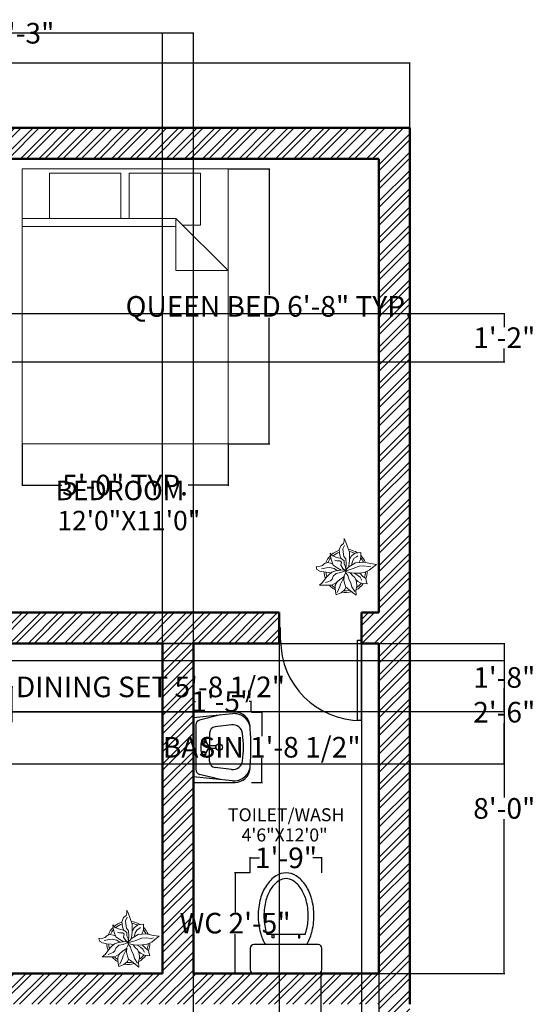
# Model space of a CAD drawing. Units: inches. Extents: x -71 to 434, y -519 to 67.
# Tile 7 of 7: x 270 to 420, y -224 to 62. Entities that reach past the tile are written whole.
import ezdxf

# ---------------------------------------------------------------- set-up
doc = ezdxf.new("R2010")
doc.units = ezdxf.units.IN
doc.header["$MEASUREMENT"] = 0
for name, color, linetype, lineweight in [('A-ANNO-DIMS', 7, 'Continuous', 18), ('A-AREA-IDEN', 7, 'Continuous', 25), ('A-FLOR-FIXT', 9, 'Continuous', 18), ('A-WALL-PATT', 8, 'Continuous', 13), ('CAY', 94, 'Continuous', 13), ('DOOR', 3, 'Continuous', 25), ('FURNITURE', 5, 'Continuous', 18), ('WALL', 50, 'Continuous', 50)]:
    doc.layers.add(name, color=color, linetype=linetype, lineweight=lineweight)
doc.layers.add('THIET-BI', color=21, linetype='Continuous')
doc.styles.add('ATT', font='romans.shx')
doc.styles.get("Standard").update_dxf_attribs({"font": 'arial.ttf'})
doc.dimstyles.get("Standard").update_dxf_attribs({"dimtxt": 6, "dimasz": 0.18, "dimexe": 0.18, "dimexo": 0.0625, "dimgap": 0.09, "dimtad": 0, "dimtih": 1, "dimtoh": 1, "dimdec": 0, "dimzin": 0, "dimdsep": 46, "dimlunit": 3, "dimtxsty": 'Standard', "dimcen": 0.09, "dimadec": 0, "dimazin": 0, "dimtfac": 1, "dimtdec": 0, "dimtofl": 0, "dimtmove": 0, "dimatfit": 3, "dimfxl": 1, "dimtolj": 1, "dimtzin": 0, "dimarcsym": 0})

# ---------------------------------------------------------------- blocks, each defined once
blk = doc.blocks.new('Bed - Queen')
for p, q in [((0, -80.00003), (0, 0)), ((0, 0), (59.99999, 0)), ((59.99999, 0), (59.99999, -80.00003)), ((7.99999, -1.2), (28.79998, -1.2)), ((7.99999, -14.4), (7.99999, -1.2)), ((28.79998, -1.2), (28.79998, -14.4)), ((31.19999, -1.2), (51.99999, -1.2)), ((31.19999, -14.4), (31.19999, -1.2)), ((51.99999, -1.2), (51.99999, -16.4)), ((0, -14.4), (44.8, -14.4)), ((44.8, -16.8), (0, -16.8)), ((59.99999, -29.6), (44.8, -14.4)), ((44.8, -14.4), (44.8, -29.6)), ((51.99999, -16.4), (46.79936, -16.4)), ((44.8, -29.6), (59.99999, -29.6)), ((59.99999, -80.00003), (0, -80.00003))]:
    blk.add_line(p, q)
blk = doc.blocks.new('A$C793314D9')
at = {"layer": 'THIET-BI'}
for p, q in [((475, 700), (25, 700)), ((0, 675), (0, 525)), ((500, 525), (500, 675)), ((25, 500), (475, 500)), ((117.1, 430), (382.9, 430)), ((163.6, 452.4), (153.8, 452.4)), ((153.8, 452.4), (153.8, 429.9)), ((153.8, 429.9), (163.6, 429.9)), ((163.6, 429.9), (163.6, 452.4)), ((336.2, 452.4), (345.9, 452.4)), ((336.2, 429.9), (336.2, 452.4)), ((345.9, 429.9), (336.2, 429.9)), ((345.9, 452.4), (345.9, 429.9))]:
    blk.add_line(p, q, dxfattribs=at)
for centre, radius, start, end in [((25, 675), 25, 90, 180), ((475, 675), 25, 0, 90), ((25, 525), 25, 180, 270), ((383.8, 333.9), 323.5, 149.09657, 164.92686), ((116.2, 333.9), 323.5, 15.07314, 30.90343), ((475, 525), 25, 270, 0), ((513.7, 298.9), 458.1, 164.92686, 180), ((383.8, 333.9), 283.5, 160.17598, 164.92686), ((116.2, 333.9), 283.5, 15.07314, 19.82402), ((-13.7, 298.9), 458.1, 0, 15.07314), ((513.7, 298.9), 418.1, 164.92686, 180), ((-13.7, 298.9), 418.1, 0, 15.07314), ((513.7, 298.9), 458.1, 180, 195.07314), ((513.7, 298.9), 418.1, 180, 195.07314), ((-13.7, 298.9), 418.1, 344.92686, 360), ((-13.7, 298.9), 458.1, 344.92686, 0), ((383.8, 263.9), 323.5, 195.07314, 213.03155), ((383.8, 263.9), 283.5, 195.07314, 213.03155), ((116.2, 263.9), 283.5, 326.96845, 344.92686), ((116.2, 263.9), 323.5, 326.96845, 344.92686), ((301.7, 210.5), 225.5, 213.03155, 237.50023), ((301.7, 210.5), 185.5, 213.03155, 237.50023), ((198.3, 210.5), 185.5, 302.49977, 326.96845), ((198.3, 210.5), 225.5, 302.49977, 326.96845), ((250, 129.3), 129.3, 237.50023, 270), ((250, 129.3), 89.3, 237.50023, 270), ((250, 129.3), 89.3, 270, 302.49977), ((250, 129.3), 129.3, 270, 302.49977)]:
    blk.add_arc(centre, radius, start, end, dxfattribs=at)
blk = doc.blocks.new('TAM')
for p, q in [((-68.4, 12), (-49.4, 25.8)), ((-61.2, -10.4), (-68.4, 12)), ((-59.4, 6.8), (-61.2, 6.8)), ((-49.4, 25.8), (-30.4, 12)), ((-30.4, 12), (-37.6, -10.4)), ((50.6, 25.8), (31.6, 12)), ((31.6, 12), (38.8, -10.4)), ((69.6, 12), (50.6, 25.8)), ((60.6, 6.8), (62.4, 6.8)), ((62.4, -10.4), (69.6, 12)), ((-59.4, -10.4), (-49.4, -10.4)), ((-9.4, -60.4), (-9.4, -50.4)), ((-9.4, -90.4), (-9.4, -60.4)), ((10.6, -60.4), (10.6, -50.4)), ((10.6, -90.4), (10.6, -60.4)), ((62.4, -10.4), (50.6, -10.4)), ((-9.4, -90.4), (10.6, -90.4))]:
    blk.add_line(p, q)
for centre in [(-49.8, 6.8), (51, 6.8)]:
    blk.add_circle(centre, 10.4)
for centre, radius, start, end in [((0.6, -221.7), 252.5, 78.57881, 101.42119), ((-49.4, -50.4), 40, 0, 90), ((50.6, -50.4), 40, 90, 180)]:
    blk.add_arc(centre, radius, start, end)
blk = doc.blocks.new('A$C0E2F1A29')
at = {"layer": 'THIET-BI'}
for p, q in [((0, 460), (0, 126.9)), ((560, 460), (0, 460)), ((13, 148.3), (44.6, 460)), ((22.6, 242.8), (63.6, 409.5)), ((457.6, 440), (102.4, 440)), ((537.4, 242.8), (496.4, 409.5)), ((547, 148.3), (515.4, 460)), ((560, 126.9), (560, 460)), ((167.1, 330), (280, 330)), ((392.9, 330), (280, 330)), ((101.6, 155.5), (117.4, 286)), ((458.4, 155.5), (442.6, 286))]:
    blk.add_line(p, q, dxfattribs=at)
blk.add_circle((280, 253.2), 25.4, dxfattribs=at)
for centre, radius, start, end in [((102.4, 400), 40, 90, 166.19533), ((457.6, 400), 40, 13.80467, 90), ((167.1, 280), 50, 90, 173.07801), ((392.9, 280), 50, 6.92199, 90), ((120, 126.9), 120, 180, 265.03849), ((142.3, 135.2), 130, 174.2113, 265.70941), ((181, 145.9), 80, 173.07801, 263.17143), ((379, 145.9), 80, 276.82857, 6.92199), ((417.7, 135.2), 130, 274.29059, 5.7887), ((440, 126.9), 120, 274.96151, 0), ((280, 1970), 1970, 265.70941, 274.29059), ((280, 972.5), 912.5, 263.17143, 276.82857)]:
    blk.add_arc(centre, radius, start, end, dxfattribs=at)
blk.add_blockref('TAM', (279.2, 369.4), dxfattribs=at)
blk = doc.blocks.new('*U13')
for p, q in [((0, 0), (0, -6)), ((40, 0), (40, -6))]:
    blk.add_line(p, q)
blk.add_lwpolyline([(0, 0), (0, 40), (1.75, 40), (1.75, 0)], close=True)
blk.add_arc((0, 0), 40, 0, 90)
blk = doc.blocks.new('*D17')
at = {"layer": 'A-ANNO-DIMS', "color": 0, "lineweight": -2, "transparency": 16777216}
for p, q in [((-12.59, 30.9), (-12.59, 49.86)), ((-12.41, 49.68), (180.23, 49.68)), ((383.23, 49.68), (190.59, 49.68)), ((383.41, 30.9), (383.41, 49.86))]:
    blk.add_line(p, q, dxfattribs=at)
at = {"layer": 'A-ANNO-DIMS', "color": 0, "transparency": 16777216}
for points in [[(-12.41, 49.71), (-12.41, 49.65), (-12.59, 49.68)], [(383.23, 49.71), (383.23, 49.65), (383.41, 49.68)]]:
    blk.add_solid(points, dxfattribs=at)
at = {"layer": 'Defpoints', "color": 0, "transparency": 16777216}
for p in [(383.41, 49.68), (-12.59, 30.83), (383.41, 30.83)]:
    blk.add_point(p, dxfattribs=at)
at = {"layer": 'A-ANNO-DIMS', "color": 0, "transparency": 16777216, "insert": (185.41, 49.68), "char_height": 6, "attachment_point": 5}
blk.add_mtext("\\A1;33'", dxfattribs=at)
blk = doc.blocks.new('12PPLT12')
at = {"color": 0, "linetype": 'ByBlock'}
for p, q in [((-0.05, 0.632), (-0.034, 0.694)), ((-0.034, 0.694), (-0.032, 0.751)), ((-0.032, 0.751), (-0.002, 0.689)), ((-0.002, 0.689), (0.044, 0.559)), ((-0.148, 0.486), (-0.116, 0.583)), ((-0.132, 0.367), (-0.148, 0.486)), ((-0.116, 0.583), (-0.05, 0.632)), ((-0.064, 0.51), (-0.026, 0.591)), ((-0.05, 0.38), (-0.064, 0.51)), ((0.044, 0.559), (0.09, 0.432)), ((-0.349, 0.334), (-0.362, 0.415)), ((-0.362, 0.415), (-0.303, 0.35)), ((-0.332, 0.247), (-0.349, 0.334)), ((-0.289, 0.136), (-0.332, 0.247)), ((-0.303, 0.35), (-0.208, 0.312)), ((-0.205, 0.231), (-0.251, 0.247)), ((-0.208, 0.312), (-0.105, 0.29)), ((-0.137, 0.231), (-0.205, 0.231)), ((-0.097, 0.204), (-0.137, 0.231)), ((-0.108, 0.279), (-0.132, 0.367)), ((-0.105, 0.29), (-0.037, 0.236)), ((-0.043, 0.334), (-0.05, 0.38)), ((0.003, 0.279), (-0.043, 0.334)), ((-0.037, 0.236), (-0.034, 0.158)), ((0.009, 0.169), (0.003, 0.279)), ((0.09, 0.253), (0.082, 0.174)), ((0.09, 0.432), (0.09, 0.339)), ((0.09, 0.339), (0.09, 0.253)), ((0.093, 0.282), (0.134, 0.347)), ((0.155, 0.228), (0.131, 0.13)), ((0.134, 0.347), (0.22, 0.415)), ((0.193, 0.293), (0.155, 0.228)), ((0.25, 0.328), (0.193, 0.293)), ((0.22, 0.415), (0.291, 0.421)), ((0.28, 0.353), (0.25, 0.328)), ((0.291, 0.421), (0.35, 0.429)), ((0.342, 0.266), (0.304, 0.19)), ((0.348, 0.331), (0.342, 0.266)), ((0.35, 0.429), (0.348, 0.331)), ((-0.671, 0.098), (-0.687, 0.095)), ((-0.687, 0.095), (-0.666, 0.036)), ((-0.59, 0.109), (-0.671, 0.098)), ((-0.666, 0.036), (-0.601, -0.005)), ((-0.536, 0.125), (-0.59, 0.109)), ((-0.563, 0.052), (-0.441, 0.074)), ((-0.487, 0.171), (-0.536, 0.125)), ((-0.425, 0.193), (-0.487, 0.171)), ((-0.441, 0.074), (-0.373, 0.084)), ((-0.346, 0.179), (-0.425, 0.193)), ((-0.373, 0.084), (-0.27, 0.057)), ((-0.292, 0.149), (-0.346, 0.179)), ((-0.229, 0.003), (-0.324, -0.027)), ((-0.194, 0.074), (-0.289, 0.136)), ((-0.27, 0.057), (-0.186, 0.006)), ((-0.069, 0.027), (-0.229, 0.003)), ((-0.108, 0.019), (-0.194, 0.074)), ((-0.01, 0.003), (-0.121, -0.038)), ((-0.11, 0.133), (-0.097, 0.204)), ((-0.069, 0.06), (-0.11, 0.133)), ((-0.01, 0.014), (-0.069, 0.06)), ((-0.002, 0.006), (-0.069, 0.027)), ((-0.034, 0.158), (-0.007, 0.101)), ((-0.018, -0.008), (0.074, 0.098)), ((-0.01, -0.005), (0.169, 0.055)), ((0.003, 0.017), (-0.01, 0.014)), ((0.003, -0.029), (-0.01, 0.003)), ((-0.007, 0.101), (0.003, 0.017)), ((0.006, 0.027), (0.009, 0.169)), ((0.082, 0.174), (0.061, 0.082)), ((0.074, 0.098), (0.223, 0.188)), ((0.169, 0.055), (0.315, 0.109)), ((0.223, 0.188), (0.421, 0.204)), ((0.315, 0.109), (0.413, 0.117)), ((0.413, 0.117), (0.524, 0.101)), ((0.421, 0.204), (0.573, 0.171)), ((0.545, 0.017), (0.429, -0.032)), ((0.524, 0.101), (0.578, 0.114)), ((0.613, 0.074), (0.545, 0.017)), ((0.573, 0.171), (0.716, 0.152)), ((0.716, 0.152), (0.613, 0.074)), ((-0.601, -0.005), (-0.503, -0.021)), ((-0.452, -0.152), (-0.536, -0.268)), ((-0.503, -0.021), (-0.4, -0.032)), ((-0.395, -0.094), (-0.452, -0.152)), ((-0.4, -0.032), (-0.357, -0.04)), ((-0.324, -0.027), (-0.395, -0.094)), ((-0.352, -0.227), (-0.387, -0.241)), ((-0.316, -0.187), (-0.352, -0.227)), ((-0.292, -0.122), (-0.316, -0.187)), ((-0.224, -0.059), (-0.292, -0.122)), ((-0.121, -0.038), (-0.224, -0.059)), ((-0.213, -0.263), (-0.135, -0.195)), ((-0.135, -0.195), (-0.053, -0.14)), ((-0.119, -0.304), (-0.04, -0.148)), ((-0.053, -0.14), (0.003, -0.029)), ((-0.037, -0.122), (-0.04, -0.219)), ((-0.04, -0.219), (-0.021, -0.308)), ((0.082, -0.038), (-0.018, -0.008)), ((-0.007, -0.024), (0.05, -0.105)), ((0.05, -0.105), (0.071, -0.181)), ((0.071, -0.181), (0.12, -0.282)), ((0.188, -0.054), (0.082, -0.038)), ((0.112, -0.051), (0.09, -0.043)), ((0.155, -0.108), (0.112, -0.051)), ((0.212, -0.152), (0.155, -0.108)), ((0.323, -0.051), (0.188, -0.054)), ((0.247, -0.246), (0.212, -0.152)), ((0.215, -0.062), (0.282, -0.103)), ((0.234, -0.2), (0.277, -0.241)), ((0.282, -0.103), (0.334, -0.146)), ((0.429, -0.032), (0.323, -0.051)), ((0.396, -0.124), (0.326, -0.054)), ((0.334, -0.146), (0.372, -0.217)), ((0.464, -0.176), (0.396, -0.124)), ((0.48, -0.257), (0.464, -0.176)), ((-0.536, -0.268), (-0.606, -0.328)), ((-0.606, -0.328), (-0.522, -0.328)), ((-0.522, -0.328), (-0.324, -0.325)), ((-0.387, -0.241), (-0.465, -0.268)), ((-0.324, -0.325), (-0.213, -0.263)), ((-0.244, -0.33), (-0.247, -0.406)), ((-0.247, -0.406), (-0.233, -0.471)), ((-0.193, -0.236), (-0.244, -0.33)), ((-0.199, -0.494), (-0.139, -0.358)), ((-0.139, -0.358), (-0.119, -0.304)), ((-0.102, -0.503), (-0.017, -0.432)), ((-0.021, -0.308), (0.006, -0.376)), ((-0.017, -0.432), (0.003, -0.378)), ((0.006, -0.376), (0.074, -0.428)), ((0.074, -0.428), (0.158, -0.496)), ((0.12, -0.282), (0.139, -0.363)), ((0.139, -0.363), (0.212, -0.474)), ((0.236, -0.444), (0.261, -0.349)), ((0.242, -0.561), (0.236, -0.444)), ((0.261, -0.349), (0.247, -0.246)), ((0.277, -0.241), (0.372, -0.287)), ((0.372, -0.287), (0.494, -0.301)), ((0.494, -0.301), (0.48, -0.257)), ((-0.233, -0.471), (-0.222, -0.551)), ((-0.222, -0.551), (-0.148, -0.522)), ((-0.148, -0.522), (-0.102, -0.503)), ((0.158, -0.496), (0.242, -0.561))]:
    blk.add_line(p, q, dxfattribs=at)
for radius, start, end in [(0.5, 107.123, 130.9816), (0.5, 56.9563, 82.295), (0.5, 134.8021, 159.1804), (0.458, 138.4756, 155.3347), (0.458, 107.9864, 130.5771), (0.458, 62.6899, 79.5345), (0.458, 26.2761, 41.1349), (0.5, 22.9768, 45.8473), (0.5, 182.503, 200.4563), (0.458, 183.2699, 197.4002), (0.458, 340.6559, 357.5057), (0.5, 338.5862, 359.7442), (0.5, 220.6606, 241.3393), (0.458, 225.0835, 237.5023), (0.458, 264.1886, 282.4028), (0.5, 298.3455, 324.4541), (0.458, 303.3868, 322.0756), (0.5, 259.7038, 286.1281)]:
    blk.add_arc((0, 0), radius, start, end, dxfattribs=at)
at = {"color": 0, "linetype": 'ByBlock', "style": 'ATT'}
for tag, p, flags in [('ITEM', (-1, -3.25), 3), ('ROOM_NUMBER', (-1, -4.583), 1)]:
    blk.add_attdef(tag, p, '', height=1, dxfattribs=dict(at, flags=flags))
blk = doc.blocks.new('*D24')
at = {"layer": 'A-ANNO-DIMS', "color": 0, "lineweight": -2, "transparency": 16777216}
for p, q in [((330.58, 18.91), (342.7, 18.91)), ((342.52, 18.73), (342.52, -17.71)), ((342.52, -60.91), (342.52, -24.46)), ((330.58, -61.09), (342.7, -61.09))]:
    blk.add_line(p, q, dxfattribs=at)
at = {"layer": 'A-ANNO-DIMS', "color": 0, "transparency": 16777216}
for points in [[(342.49, 18.73), (342.55, 18.73), (342.52, 18.91)], [(342.49, -60.91), (342.55, -60.91), (342.52, -61.09)]]:
    blk.add_solid(points, dxfattribs=at)
at = {"layer": 'Defpoints', "color": 0, "transparency": 16777216}
for p in [(330.52, 18.91), (342.52, 18.91), (330.52, -61.09)]:
    blk.add_point(p, dxfattribs=at)
at = {"layer": 'A-ANNO-DIMS', "color": 0, "transparency": 16777216, "insert": (342.52, -21.09), "char_height": 6, "attachment_point": 5}
blk.add_mtext('\\A1;QUEEN BED 6\'-8" TYP.', dxfattribs=at)
blk = doc.blocks.new('*D25')
at = {"layer": 'A-ANNO-DIMS', "color": 0, "lineweight": -2, "transparency": 16777216}
for p, q in [((270.52, -61.15), (270.52, -73.27)), ((330.52, -61.15), (330.52, -73.27)), ((270.7, -73.09), (282.14, -73.09)), ((330.34, -73.09), (318.9, -73.09))]:
    blk.add_line(p, q, dxfattribs=at)
at = {"layer": 'A-ANNO-DIMS', "color": 0, "transparency": 16777216}
for points in [[(270.7, -73.06), (270.7, -73.12), (270.52, -73.09)], [(330.34, -73.06), (330.34, -73.12), (330.52, -73.09)]]:
    blk.add_solid(points, dxfattribs=at)
at = {"layer": 'Defpoints', "color": 0, "transparency": 16777216}
for p in [(270.52, -61.09), (330.52, -61.09), (330.52, -73.09)]:
    blk.add_point(p, dxfattribs=at)
at = {"layer": 'A-ANNO-DIMS', "color": 0, "transparency": 16777216, "insert": (300.52, -73.09), "char_height": 6, "attachment_point": 5}
blk.add_mtext('\\A1;5\'-0" TYP.', dxfattribs=at)
blk = doc.blocks.new('*D28')
at = {"layer": 'A-ANNO-DIMS', "color": 0, "lineweight": -2, "transparency": 16777216}
for p, q in [((336.91, -185.93), (332.4, -185.93)), ((332.58, -186.11), (332.58, -197.36)), ((332.58, -214.99), (332.58, -203.74)), ((336.91, -215.17), (332.4, -215.17))]:
    blk.add_line(p, q, dxfattribs=at)
at = {"layer": 'A-ANNO-DIMS', "color": 0, "transparency": 16777216}
for points in [[(332.55, -186.11), (332.61, -186.11), (332.58, -185.93)], [(332.55, -214.99), (332.61, -214.99), (332.58, -215.17)]]:
    blk.add_solid(points, dxfattribs=at)
at = {"layer": 'Defpoints', "color": 0, "transparency": 16777216}
for p in [(336.97, -185.93), (332.58, -215.17), (336.97, -215.17)]:
    blk.add_point(p, dxfattribs=at)
at = {"layer": 'A-ANNO-DIMS', "color": 0, "transparency": 16777216, "insert": (332.58, -200.55), "char_height": 6, "attachment_point": 5}
blk.add_mtext('\\A1;WC 2\'-5"', dxfattribs=at)
blk = doc.blocks.new('*D29')
at = {"layer": 'A-ANNO-DIMS', "color": 0, "lineweight": -2, "transparency": 16777216}
for p, q in [((336.97, -185.87), (336.97, -181.37)), ((337.15, -181.55), (339.63, -181.55)), ((357.67, -181.55), (355.19, -181.55)), ((357.85, -185.87), (357.85, -181.37))]:
    blk.add_line(p, q, dxfattribs=at)
at = {"layer": 'A-ANNO-DIMS', "color": 0, "transparency": 16777216}
for points in [[(337.15, -181.52), (337.15, -181.58), (336.97, -181.55)], [(357.67, -181.52), (357.67, -181.58), (357.85, -181.55)]]:
    blk.add_solid(points, dxfattribs=at)
at = {"layer": 'Defpoints', "color": 0, "transparency": 16777216}
for p in [(336.97, -181.55), (336.97, -185.93), (357.85, -185.93)]:
    blk.add_point(p, dxfattribs=at)
at = {"layer": 'A-ANNO-DIMS', "color": 0, "transparency": 16777216, "insert": (347.41, -181.55), "char_height": 6, "attachment_point": 5}
blk.add_mtext('\\A1;1\'-9"', dxfattribs=at)
blk = doc.blocks.new('*D34')
at = {"layer": 'A-ANNO-DIMS', "color": 0, "lineweight": -2, "transparency": 16777216}
for p, q in [((337.32, -139.15), (340.51, -139.15)), ((340.33, -139.33), (340.33, -146.17)), ((340.33, -159.4), (340.33, -152.56)), ((337.32, -159.58), (340.51, -159.58))]:
    blk.add_line(p, q, dxfattribs=at)
at = {"layer": 'A-ANNO-DIMS', "color": 0, "transparency": 16777216}
for points in [[(340.3, -139.33), (340.36, -139.33), (340.33, -139.15)], [(340.3, -159.4), (340.36, -159.4), (340.33, -159.58)]]:
    blk.add_solid(points, dxfattribs=at)
at = {"layer": 'Defpoints', "color": 0, "transparency": 16777216}
for p in [(337.26, -139.15), (340.33, -139.15), (337.26, -159.58)]:
    blk.add_point(p, dxfattribs=at)
at = {"layer": 'A-ANNO-DIMS', "color": 0, "transparency": 16777216, "insert": (340.33, -149.37), "char_height": 6, "attachment_point": 5}
blk.add_mtext('\\A1;BASIN 1\'-8 1/2"', dxfattribs=at)
blk = doc.blocks.new('*D35')
at = {"layer": 'A-ANNO-DIMS', "color": 0, "lineweight": -2, "transparency": 16777216}
for p, q in [((320.41, -139.09), (320.41, -135.9)), ((320.59, -136.08), (321.05, -136.08)), ((337.08, -136.08), (336.62, -136.08)), ((337.26, -139.09), (337.26, -135.9))]:
    blk.add_line(p, q, dxfattribs=at)
at = {"layer": 'A-ANNO-DIMS', "color": 0, "transparency": 16777216}
for points in [[(320.59, -136.05), (320.59, -136.11), (320.41, -136.08)], [(337.08, -136.05), (337.08, -136.11), (337.26, -136.08)]]:
    blk.add_solid(points, dxfattribs=at)
at = {"layer": 'Defpoints', "color": 0, "transparency": 16777216}
for p in [(320.41, -136.08), (320.41, -139.15), (337.26, -139.15)]:
    blk.add_point(p, dxfattribs=at)
at = {"layer": 'A-ANNO-DIMS', "color": 0, "transparency": 16777216, "insert": (328.83, -136.08), "char_height": 6, "attachment_point": 5}
blk.add_mtext('\\A1;1\'-5"', dxfattribs=at)
blk = doc.blocks.new('*D42')
at = {"layer": 'A-ANNO-DIMS', "color": 0, "lineweight": -2, "transparency": 16777216}
for p, q in [((199.01, -142.05), (199.01, -131.63)), ((267.7, -142.05), (267.7, -131.63)), ((199.19, -131.81), (267.52, -131.81)), ((267.7, -131.81), (267.88, -131.81))]:
    blk.add_line(p, q, dxfattribs=at)
at = {"layer": 'A-ANNO-DIMS', "color": 0, "transparency": 16777216}
for points in [[(199.19, -131.78), (199.19, -131.84), (199.01, -131.81)], [(267.52, -131.78), (267.52, -131.84), (267.7, -131.81)]]:
    blk.add_solid(points, dxfattribs=at)
at = {"layer": 'Defpoints', "color": 0, "transparency": 16777216}
for p in [(267.7, -131.81), (199.01, -142.12), (267.7, -142.12)]:
    blk.add_point(p, dxfattribs=at)
at = {"layer": 'A-ANNO-DIMS', "color": 0, "transparency": 16777216, "insert": (307.94, -131.81), "char_height": 6, "attachment_point": 5}
blk.add_mtext('\\A1;DINING SET 5\'-8 1/2"', dxfattribs=at)
blk = doc.blocks.new('*D49')
at = {"layer": 'A-ANNO-DIMS', "color": 0, "lineweight": -2, "transparency": 16777216}
for p, q in [((221.41, -473.1), (221.41, 58.56)), ((221.59, 58.38), (262.84, 58.38)), ((320.23, 58.38), (278.98, 58.38)), ((320.41, -473.1), (320.41, 58.56))]:
    blk.add_line(p, q, dxfattribs=at)
at = {"layer": 'A-ANNO-DIMS', "color": 0, "transparency": 16777216}
for points in [[(221.59, 58.41), (221.59, 58.35), (221.41, 58.38)], [(320.23, 58.41), (320.23, 58.35), (320.41, 58.38)]]:
    blk.add_solid(points, dxfattribs=at)
at = {"layer": 'Defpoints', "color": 0, "transparency": 16777216}
for p in [(320.41, 58.38), (221.41, -473.17), (320.41, -473.17)]:
    blk.add_point(p, dxfattribs=at)
at = {"layer": 'A-ANNO-DIMS', "color": 0, "transparency": 16777216, "insert": (270.91, 58.38), "char_height": 6, "attachment_point": 5}
blk.add_mtext('\\A1;8\'-3"', dxfattribs=at)
blk = doc.blocks.new('*D53')
at = {"layer": 'A-ANNO-DIMS', "color": 0, "lineweight": -2, "transparency": 16777216}
for p, q in [((374.47, -119.17), (411.14, -119.17)), ((410.96, -119.35), (410.96, -164.01)), ((410.96, -214.99), (410.96, -170.32)), ((374.47, -215.17), (411.14, -215.17))]:
    blk.add_line(p, q, dxfattribs=at)
at = {"layer": 'A-ANNO-DIMS', "color": 0, "transparency": 16777216}
for points in [[(410.93, -119.35), (410.99, -119.35), (410.96, -119.17)], [(410.93, -214.99), (410.99, -214.99), (410.96, -215.17)]]:
    blk.add_solid(points, dxfattribs=at)
at = {"layer": 'Defpoints', "color": 0, "transparency": 16777216}
for p in [(374.41, -119.17), (374.41, -215.17), (410.96, -215.17)]:
    blk.add_point(p, dxfattribs=at)
at = {"layer": 'A-ANNO-DIMS', "color": 0, "transparency": 16777216, "insert": (410.96, -167.17), "char_height": 6, "attachment_point": 5}
blk.add_mtext('\\A1;8\'-0"', dxfattribs=at)
blk = doc.blocks.new('*D55')
at = {"layer": 'A-ANNO-DIMS', "color": 0, "lineweight": -2, "transparency": 16777216}
for p, q in [((345.41, -119.23), (345.41, -509.9)), ((369.41, -119.23), (369.41, -509.9)), ((345.59, -509.72), (349.29, -509.72)), ((369.23, -509.72), (365.52, -509.72))]:
    blk.add_line(p, q, dxfattribs=at)
at = {"layer": 'A-ANNO-DIMS', "color": 0, "transparency": 16777216}
for points in [[(345.59, -509.69), (345.59, -509.75), (345.41, -509.72)], [(369.23, -509.69), (369.23, -509.75), (369.41, -509.72)]]:
    blk.add_solid(points, dxfattribs=at)
at = {"layer": 'Defpoints', "color": 0, "transparency": 16777216}
for p in [(345.41, -119.17), (369.41, -119.17), (369.41, -509.72)]:
    blk.add_point(p, dxfattribs=at)
at = {"layer": 'A-ANNO-DIMS', "color": 0, "transparency": 16777216, "insert": (357.41, -509.72), "char_height": 6, "attachment_point": 5}
blk.add_mtext('\\A1;2\'-0"', dxfattribs=at)
blk = doc.blocks.new('*D57')
at = {"layer": 'A-ANNO-DIMS', "color": 0, "lineweight": -2, "transparency": 16777216}
for p, q in [((149.47, -124.17), (411.14, -124.17)), ((410.96, -124.35), (410.96, -136.01)), ((410.96, -153.99), (410.96, -142.32)), ((149.47, -154.17), (411.14, -154.17))]:
    blk.add_line(p, q, dxfattribs=at)
at = {"layer": 'A-ANNO-DIMS', "color": 0, "transparency": 16777216}
for points in [[(410.93, -124.35), (410.99, -124.35), (410.96, -124.17)], [(410.93, -153.99), (410.99, -153.99), (410.96, -154.17)]]:
    blk.add_solid(points, dxfattribs=at)
at = {"layer": 'Defpoints', "color": 0, "transparency": 16777216}
for p in [(149.41, -124.17), (149.41, -154.17), (410.96, -154.17)]:
    blk.add_point(p, dxfattribs=at)
at = {"layer": 'A-ANNO-DIMS', "color": 0, "transparency": 16777216, "insert": (410.96, -139.17), "char_height": 6, "attachment_point": 5}
blk.add_mtext('\\A1;2\'-6"', dxfattribs=at)
blk = doc.blocks.new('*D61')
at = {"layer": 'A-ANNO-DIMS', "color": 0, "lineweight": -2, "transparency": 16777216}
for p, q in [((221.47, -23.17), (411.14, -23.17)), ((410.96, -23.35), (410.96, -27.11)), ((410.96, -37.08), (410.96, -33.32)), ((220.39, -37.26), (411.14, -37.26))]:
    blk.add_line(p, q, dxfattribs=at)
at = {"layer": 'A-ANNO-DIMS', "color": 0, "transparency": 16777216}
for points in [[(410.93, -23.35), (410.99, -23.35), (410.96, -23.17)], [(410.93, -37.08), (410.99, -37.08), (410.96, -37.26)]]:
    blk.add_solid(points, dxfattribs=at)
at = {"layer": 'Defpoints', "color": 0, "transparency": 16777216}
for p in [(221.41, -23.17), (220.33, -37.26), (410.96, -37.26)]:
    blk.add_point(p, dxfattribs=at)
at = {"layer": 'A-ANNO-DIMS', "color": 0, "transparency": 16777216, "insert": (410.96, -30.21), "char_height": 6, "attachment_point": 5}
blk.add_mtext('\\A1;1\'-2"', dxfattribs=at)
blk = doc.blocks.new('*D63')
at = {"layer": 'A-ANNO-DIMS', "color": 0, "lineweight": -2, "transparency": 16777216}
for p, q in [((369.41, -119.23), (369.41, -509.9)), ((374.41, -119.23), (374.41, -509.9)), ((369.41, -509.72), (369.23, -509.72)), ((374.23, -509.72), (369.59, -509.72))]:
    blk.add_line(p, q, dxfattribs=at)
at = {"layer": 'A-ANNO-DIMS', "color": 0, "transparency": 16777216}
for points in [[(369.59, -509.69), (369.59, -509.75), (369.41, -509.72)], [(374.23, -509.69), (374.23, -509.75), (374.41, -509.72)]]:
    blk.add_solid(points, dxfattribs=at)
at = {"layer": 'Defpoints', "color": 0, "transparency": 16777216}
for p in [(369.41, -119.17), (374.41, -119.17), (369.41, -509.72)]:
    blk.add_point(p, dxfattribs=at)
at = {"layer": 'A-ANNO-DIMS', "color": 0, "transparency": 16777216, "insert": (361.16, -509.72), "char_height": 6, "attachment_point": 5}
blk.add_mtext('\\A1;0\'-5"', dxfattribs=at)
blk = doc.blocks.new('*D64')
at = {"layer": 'A-ANNO-DIMS', "color": 0, "lineweight": -2, "transparency": 16777216}
for p, q in [((320.35, -119.17), (-40.32, -119.17)), ((-40.14, -119.35), (-40.14, -126)), ((-40.14, -138.97), (-40.14, -132.31)), ((320.35, -139.15), (-40.32, -139.15))]:
    blk.add_line(p, q, dxfattribs=at)
at = {"layer": 'A-ANNO-DIMS', "color": 0, "transparency": 16777216}
for points in [[(-40.17, -119.35), (-40.11, -119.35), (-40.14, -119.17)], [(-40.17, -138.97), (-40.11, -138.97), (-40.14, -139.15)]]:
    blk.add_solid(points, dxfattribs=at)
at = {"layer": 'Defpoints', "color": 0, "transparency": 16777216}
for p in [(320.41, -119.17), (-40.14, -139.15), (320.41, -139.15)]:
    blk.add_point(p, dxfattribs=at)
at = {"layer": 'A-ANNO-DIMS', "color": 0, "transparency": 16777216, "insert": (-40.14, -129.16), "char_height": 6, "attachment_point": 5}
blk.add_mtext('\\A1;1\'-8"', dxfattribs=at)
blk = doc.blocks.new('*D65')
at = {"layer": 'A-ANNO-DIMS', "color": 0, "lineweight": -2, "transparency": 16777216}
for p, q in [((357.54, -214.92), (357.54, -509.9)), ((374.41, -215.23), (374.41, -509.9)), ((357.72, -509.72), (358.19, -509.72)), ((374.23, -509.72), (373.76, -509.72))]:
    blk.add_line(p, q, dxfattribs=at)
at = {"layer": 'A-ANNO-DIMS', "color": 0, "transparency": 16777216}
for points in [[(357.72, -509.69), (357.72, -509.75), (357.54, -509.72)], [(374.23, -509.69), (374.23, -509.75), (374.41, -509.72)]]:
    blk.add_solid(points, dxfattribs=at)
at = {"layer": 'Defpoints', "color": 0, "transparency": 16777216}
for p in [(357.54, -214.86), (374.41, -215.17), (374.41, -509.72)]:
    blk.add_point(p, dxfattribs=at)
at = {"layer": 'A-ANNO-DIMS', "color": 0, "transparency": 16777216, "insert": (365.97, -509.72), "char_height": 6, "attachment_point": 5}
blk.add_mtext('\\A1;1\'-5"', dxfattribs=at)
blk = doc.blocks.new('*D67')
at = {"layer": 'A-ANNO-DIMS', "color": 0, "lineweight": -2, "transparency": 16777216}
for p, q in [((107.56, -119.17), (411.14, -119.17)), ((410.96, -119.35), (410.96, -125.92)), ((410.96, -138.8), (410.96, -132.22)), ((107.56, -138.98), (411.14, -138.98))]:
    blk.add_line(p, q, dxfattribs=at)
at = {"layer": 'A-ANNO-DIMS', "color": 0, "transparency": 16777216}
for points in [[(410.93, -119.35), (410.99, -119.35), (410.96, -119.17)], [(410.93, -138.8), (410.99, -138.8), (410.96, -138.98)]]:
    blk.add_solid(points, dxfattribs=at)
at = {"layer": 'Defpoints', "color": 0, "transparency": 16777216}
for p in [(107.49, -119.17), (107.49, -138.98), (410.96, -138.98)]:
    blk.add_point(p, dxfattribs=at)
at = {"layer": 'A-ANNO-DIMS', "color": 0, "transparency": 16777216, "insert": (410.96, -129.07), "char_height": 6, "attachment_point": 5}
blk.add_mtext('\\A1;1\'-8"', dxfattribs=at)
blk = doc.blocks.new('*D69')
at = {"layer": 'A-ANNO-DIMS', "color": 0, "lineweight": -2, "transparency": 16777216}
for p, q in [((149.41, -215.1), (149.41, 58.56)), ((149.59, 58.38), (220.29, 58.38)), ((311.23, 58.38), (240.52, 58.38)), ((311.41, -215.1), (311.41, 58.56))]:
    blk.add_line(p, q, dxfattribs=at)
at = {"layer": 'A-ANNO-DIMS', "color": 0, "transparency": 16777216}
for points in [[(149.59, 58.41), (149.59, 58.35), (149.41, 58.38)], [(311.23, 58.41), (311.23, 58.35), (311.41, 58.38)]]:
    blk.add_solid(points, dxfattribs=at)
at = {"layer": 'Defpoints', "color": 0, "transparency": 16777216}
for p in [(311.41, 58.38), (149.41, -215.17), (311.41, -215.17)]:
    blk.add_point(p, dxfattribs=at)
at = {"layer": 'A-ANNO-DIMS', "color": 0, "transparency": 16777216, "insert": (230.41, 58.38), "char_height": 6, "attachment_point": 5}
blk.add_mtext('\\A1;13\'-6"', dxfattribs=at)

msp = doc.modelspace()

# ---------------------------------------------------------------- hatches: boundary and pattern name
at = {"layer": 'A-WALL-PATT'}
h = msp.add_hatch(dxfattribs=at)
h.set_pattern_fill('ANSI32', color=256, scale=10)
h.set_pattern_definition([(45, (-213.138, 0), (-2.65165, 2.65165), []), (45, (-211.37, 0), (-2.65165, 2.65165), [])])
h.paths.add_polyline_path([(383.41, 30.83), (230.41, 30.83), (149.41, 30.83), (-12.59, 30.83), (-12.59, -20.17), (-3.59, -20.17), (-3.59, 21.83), (140.41, 21.83), (140.41, 15.83), (149.41, 15.83), (149.41, 21.83), (221.41, 21.83), (221.41, 15.83), (230.41, 15.83), (230.41, 21.83), (374.41, 21.83), (374.41, -110.17), (369.41, -110.17), (369.41, -119.17), (374.41, -119.17), (374.41, -215.17), (320.41, -215.17), (320.41, -119.17), (345.41, -119.17), (345.41, -110.17), (221.41, -110.17), (221.41, -119.17), (311.41, -119.17), (311.41, -215.17), (192.42, -215.17), (192.42, -224.17), (221.41, -224.17), (221.41, -228.23), (230.41, -228.23), (230.41, -224.17), (374.41, -224.17), (374.41, -368.17), (230.41, -368.17), (230.41, -266.34), (221.41, -266.34), (221.41, -368.17), (192.08, -368.17), (192.08, -377.17), (230.41, -377.17), (374.41, -377.17), (374.41, -473.17), (230.41, -473.17), (212.41, -473.17), (212.41, -482.17), (383.41, -482.17), (383.41, -377.17), (383.41, -224.17), (383.41, -119.17)])
h.paths.add_polyline_path([(149.41, -110.17), (-3.59, -110.17), (-3.59, -68.17), (-12.59, -68.17), (-12.59, -276.67), (-3.59, -276.67), (-3.59, -224.17), (154.41, -224.17), (154.41, -215.17), (149.41, -215.17), (149.41, -154.17), (140.41, -154.17), (140.41, -215.17), (-3.59, -215.17), (-3.59, -119.17), (19.82, -119.17), (140.41, -119.17), (140.41, -124.17), (149.41, -124.17)])
h.paths.add_polyline_path([(84.91, -368.17), (-3.59, -368.17), (-3.59, -324.67), (-12.59, -324.67), (-12.59, -377.17), (-12.59, -401.17), (-3.59, -401.17), (-3.59, -377.17), (84.91, -377.17)], flags=17)
h.paths.add_polyline_path([(1.41, -473.17), (-3.59, -473.17), (-3.59, -468.17), (-12.59, -468.17), (-12.59, -482.17), (1.41, -482.17)], flags=17)

# ---------------------------------------------------------------- linework, layer by layer
at = {"layer": 'DOOR'}
for p, q in [((345.82, -114.67), (345.41, -114.67)), ((369.26, -114.67), (369.41, -114.67))]:
    msp.add_line(p, q, dxfattribs=at)
at = {"layer": 'WALL'}
for p, q in [((230.41, 30.83), (383.41, 30.83)), ((383.41, 30.83), (383.41, -119.17)), ((230.41, 21.83), (374.41, 21.83)), ((374.41, 21.83), (374.41, -110.17)), ((345.41, -110.17), (221.41, -110.17)), ((345.41, -110.17), (345.41, -119.17)), ((374.41, -110.17), (369.41, -110.17)), ((369.41, -110.17), (369.41, -119.17)), ((311.41, -119.17), (221.41, -119.17)), ((311.41, -119.17), (311.41, -215.17)), ((320.41, -119.17), (320.41, -215.17)), ((345.41, -119.17), (320.41, -119.17)), ((374.41, -119.17), (369.41, -119.17)), ((374.41, -119.17), (374.41, -215.17)), ((383.41, -119.17), (383.41, -224.17)), ((192.42, -215.17), (311.41, -215.17)), ((320.41, -215.17), (374.41, -215.17))]:
    msp.add_line(p, q, dxfattribs=at)

# ---------------------------------------------------------------- block references
at = {"layer": 'A-FLOR-FIXT'}
for name, p, xscale, yscale, zscale, rotation in [('A$C0E2F1A29', (337.19, -159.58), 0.0364928073733764, 0.0364928073733764, 0.0364928073733764, 90), ('A$C793314D9', (357.85, -185.93), 0.0417598062073127, 0.0417598062073127, 0.0417598062073127, 180)]:
    msp.add_blockref(name, p, dxfattribs=dict(at, xscale=xscale, yscale=yscale, zscale=zscale, rotation=rotation))
at = {"layer": 'CAY', "xscale": 12.58515090877727, "yscale": 12.58515090877727, "zscale": 12.58515090877727}
for p in [(364.78, -98.08), (301.49, -206.26)]:
    msp.add_blockref('12PPLT12', p, dxfattribs=at)
at = {"layer": 'DOOR', "xscale": 0.5859930162751628, "yscale": 0.5859930162751628, "zscale": 0.5859930162751628, "rotation": 179.9999999999856}
msp.add_blockref('*U13', (369.26, -118.18), dxfattribs=at)
at = {"layer": 'FURNITURE'}
msp.add_blockref('Bed - Queen', (270.52, 18.91), dxfattribs=at)

# ---------------------------------------------------------------- texts
at = {"layer": 'A-AREA-IDEN'}
for s, height, p in [('BEDROOM', 5.643, (280.31, -77.48)), ('12\'0"X11\'0"', 5.6432, (280.81, -86.23)), ('TOILET/WASH', 3.7834, (330.49, -170.91)), ('4\'6"X12\'0"', 3.783, (334.45, -176.79))]:
    msp.add_text(s, height=height, dxfattribs=at).set_placement(p)

# ---------------------------------------------------------------- dimensions: what is measured, and where the dimension line sits
at = {"layer": 'A-ANNO-DIMS'}
for base, p1, p2, override, picture, middle in [((311.41, 58.38), (149.41, -215.17), (311.41, -215.17), {"dimdec": 1, "dimlfac": 1, "dimrnd": 0, "dimzin": 1, "dimdsep": 46, "dimlunit": 4, "dimfrac": 2}, '*D69', (230.41, 58.38)), ((320.41, 58.38), (221.41, -473.17), (320.41, -473.17), {"dimdec": 1, "dimlfac": 1, "dimrnd": 0, "dimzin": 1, "dimdsep": 46, "dimlunit": 4, "dimfrac": 2}, '*D49', (270.91, 58.38)), ((383.41, 49.68), (-12.59, 30.83), (383.41, 30.83), {"dimclrd": 0, "dimclre": 0, "dimclrt": 0}, '*D17', (185.41, 49.68)), ((369.41, -509.72), (345.41, -119.17), (369.41, -119.17), {"dimdec": 1, "dimlfac": 1, "dimrnd": 0, "dimzin": 1, "dimdsep": 46, "dimlunit": 4, "dimfrac": 2}, '*D55', (357.41, -509.72)), ((369.41, -509.72), (374.41, -119.17), (369.41, -119.17), {"dimdec": 1, "dimlfac": 1, "dimrnd": 0, "dimzin": 1, "dimdsep": 46, "dimlunit": 4, "dimfrac": 2}, '*D63', (361.16, -509.72)), ((374.41, -509.72), (357.54, -214.86), (374.41, -215.17), {"dimdec": 1, "dimlfac": 1, "dimrnd": 0, "dimzin": 1, "dimdsep": 46, "dimlunit": 4, "dimfrac": 2}, '*D65', (365.97, -509.72))]:
    dim = msp.add_linear_dim(base=base, p1=p1, p2=p2, dimstyle='Standard', override=override, dxfattribs=at)
    dim.commit()
    dim.dimension.update_dxf_attribs({"geometry": picture, "text_midpoint": middle})
for base, p1, p2, angle, text, picture, middle in [((342.52, 18.91), (330.52, -61.09), (330.52, 18.91), 90, 'QUEEN BED <> TYP.', '*D24', (342.52, -21.09)), ((340.33, -139.15), (337.26, -159.58), (337.26, -139.15), 90, 'BASIN <>', '*D34', (340.33, -149.37)), ((332.58, -215.17), (336.97, -185.93), (336.97, -215.17), 270, 'WC <>', '*D28', (332.58, -200.55))]:
    dim = msp.add_linear_dim(base=base, p1=p1, p2=p2, angle=angle, text=text, dimstyle='Standard', override={"dimdec": 1, "dimlfac": 1, "dimrnd": 0, "dimzin": 1, "dimdsep": 46, "dimlunit": 4, "dimfrac": 2}, dxfattribs=at)
    dim.commit()
    dim.dimension.update_dxf_attribs({"geometry": picture, "text_midpoint": middle})
for base, p1, p2, angle, picture, middle in [((410.96, -37.26), (221.41, -23.17), (220.33, -37.26), 90, '*D61', (410.96, -30.21)), ((-40.14, -139.15), (320.41, -119.17), (320.41, -139.15), 90, '*D64', (-40.14, -129.16)), ((410.96, -138.98), (107.49, -119.17), (107.49, -138.98), 90, '*D67', (410.96, -129.07)), ((410.96, -215.17), (374.41, -119.17), (374.41, -215.17), 90, '*D53', (410.96, -167.17)), ((410.96, -154.17), (149.41, -124.17), (149.41, -154.17), 90, '*D57', (410.96, -139.17)), ((320.4078, -136.0824), (337.2616, -139.1478), (320.4078, -139.1478), 180, '*D35', (328.8347, -136.0824)), ((336.97, -181.55), (357.85, -185.93), (336.97, -185.93), 180, '*D29', (347.41, -181.55))]:
    dim = msp.add_linear_dim(base=base, p1=p1, p2=p2, angle=angle, dimstyle='Standard', override={"dimdec": 1, "dimlfac": 1, "dimrnd": 0, "dimzin": 1, "dimdsep": 46, "dimlunit": 4, "dimfrac": 2}, dxfattribs=at)
    dim.commit()
    dim.dimension.update_dxf_attribs({"geometry": picture, "text_midpoint": middle})
for base, p1, p2, text, picture, middle in [((330.52, -73.09), (270.52, -61.09), (330.52, -61.09), '<> TYP.', '*D25', (300.52, -73.09)), ((267.7, -131.81), (199.01, -142.12), (267.7, -142.12), 'DINING SET <>', '*D42', (307.94, -131.81))]:
    dim = msp.add_linear_dim(base=base, p1=p1, p2=p2, text=text, dimstyle='Standard', override={"dimdec": 1, "dimlfac": 1, "dimrnd": 0, "dimzin": 1, "dimdsep": 46, "dimlunit": 4, "dimfrac": 2}, dxfattribs=at)
    dim.commit()
    dim.dimension.update_dxf_attribs({"geometry": picture, "text_midpoint": middle})

doc.saveas('drawing.dxf')
